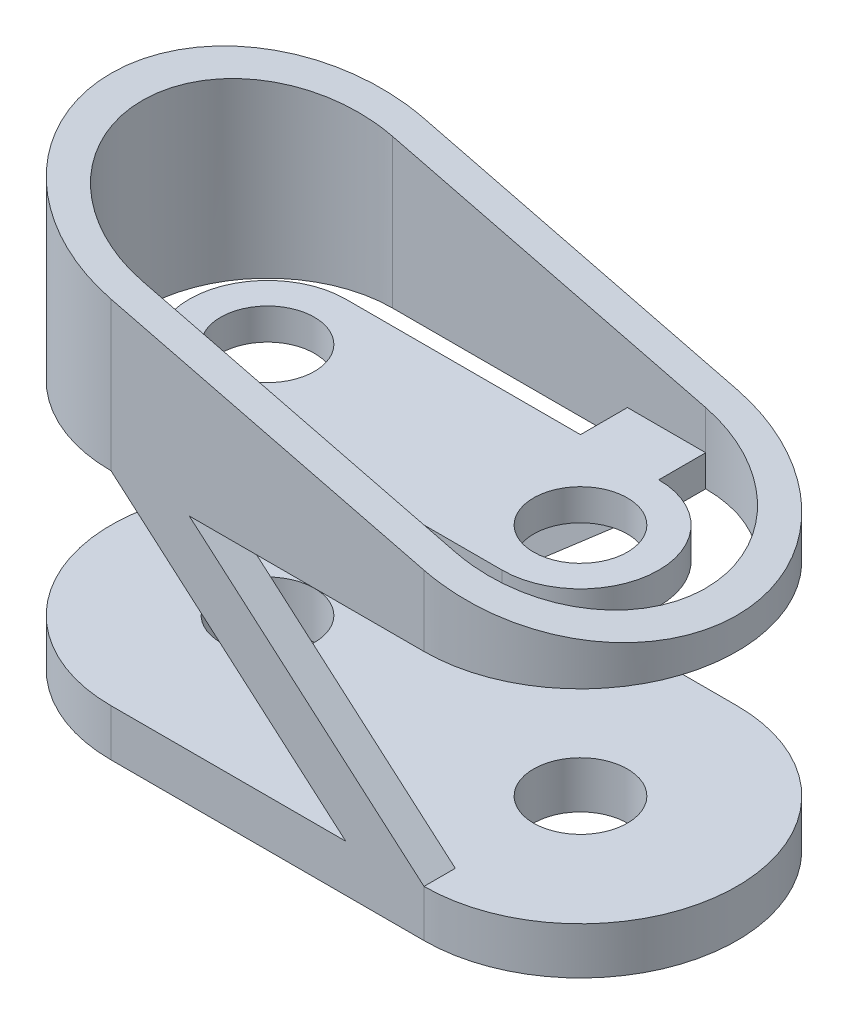
ISO-10303-21;
HEADER;
FILE_DESCRIPTION(('STEP AP214'),'2;1');
FILE_NAME('part.step','',(''),(''),'','','');
FILE_SCHEMA(('AUTOMOTIVE_DESIGN { 1 0 10303 214 1 1 1 1 }'));
ENDSEC;
DATA;
#1=APPLICATION_CONTEXT('core data for automotive mechanical design processes');
#2=APPLICATION_PROTOCOL_DEFINITION('international standard','automotive_design',2000,#1);
#3=PRODUCT_CONTEXT('',#1,'mechanical');
#4=PRODUCT('Part','Part','',(#3));
#5=PRODUCT_RELATED_PRODUCT_CATEGORY('part','',(#4));
#6=PRODUCT_DEFINITION_FORMATION('','',#4);
#7=PRODUCT_DEFINITION_CONTEXT('part definition',#1,'design');
#8=PRODUCT_DEFINITION('design','',#6,#7);
#9=PRODUCT_DEFINITION_SHAPE('','',#8);
#10=(LENGTH_UNIT() NAMED_UNIT(*) SI_UNIT(.MILLI.,.METRE.));
#11=(NAMED_UNIT(*) PLANE_ANGLE_UNIT() SI_UNIT($,.RADIAN.));
#12=(NAMED_UNIT(*) SI_UNIT($,.STERADIAN.) SOLID_ANGLE_UNIT());
#13=UNCERTAINTY_MEASURE_WITH_UNIT(LENGTH_MEASURE(1.E-05),#10,'distance_accuracy_value','');
#14=(GEOMETRIC_REPRESENTATION_CONTEXT(3) GLOBAL_UNCERTAINTY_ASSIGNED_CONTEXT((#13)) GLOBAL_UNIT_ASSIGNED_CONTEXT((#10,
#11,#12)) REPRESENTATION_CONTEXT('',''));
#15=CARTESIAN_POINT('',(0.,0.,0.));
#16=DIRECTION('',(0.,0.,1.));
#17=DIRECTION('',(1.,0.,0.));
#18=AXIS2_PLACEMENT_3D('',#15,#16,#17);
#19=CARTESIAN_POINT('',(100.,105.,-40.));
#20=DIRECTION('',(0.,0.,1.));
#21=DIRECTION('',(1.,0.,0.));
#22=AXIS2_PLACEMENT_3D('',#19,#20,#21);
#23=PLANE('',#22);
#24=DIRECTION('',(0.970142500145332,-0.242535625036333,0.));
#25=VECTOR('',#24,1.);
#26=CARTESIAN_POINT('',(99.4117647058824,102.647058823529,-40.));
#27=LINE('',#26,#25);
#28=CARTESIAN_POINT('',(0.,127.5,-40.));
#29=VERTEX_POINT('',#28);
#30=CARTESIAN_POINT('',(100.,102.5,-40.));
#31=VERTEX_POINT('',#30);
#32=EDGE_CURVE('E559',#29,#31,#27,.T.);
#33=ORIENTED_EDGE('',*,*,#32,.F.);
#34=DIRECTION('',(0.,-1.,0.));
#35=VECTOR('',#34,1.);
#36=CARTESIAN_POINT('',(0.,105.,-40.));
#37=LINE('',#36,#35);
#38=CARTESIAN_POINT('',(0.,80.,-40.));
#39=VERTEX_POINT('',#38);
#40=EDGE_CURVE('E501',#29,#39,#37,.T.);
#41=ORIENTED_EDGE('',*,*,#40,.T.);
#42=DIRECTION('',(1.,0.,0.));
#43=VECTOR('',#42,1.);
#44=CARTESIAN_POINT('',(100.,80.,-40.));
#45=LINE('',#44,#43);
#46=CARTESIAN_POINT('',(75.,80.,-40.));
#47=VERTEX_POINT('',#46);
#48=EDGE_CURVE('E494',#39,#47,#45,.T.);
#49=ORIENTED_EDGE('',*,*,#48,.T.);
#50=DIRECTION('',(0.,-1.,0.));
#51=VECTOR('',#50,1.);
#52=CARTESIAN_POINT('',(75.,105.,-40.));
#53=LINE('',#52,#51);
#54=CARTESIAN_POINT('',(75.,90.,-40.));
#55=VERTEX_POINT('',#54);
#56=EDGE_CURVE('E530',#55,#47,#53,.T.);
#57=ORIENTED_EDGE('',*,*,#56,.F.);
#58=DIRECTION('',(-1.,0.,0.));
#59=VECTOR('',#58,1.);
#60=CARTESIAN_POINT('',(0.,90.,-40.));
#61=LINE('',#60,#59);
#62=CARTESIAN_POINT('',(100.,90.,-40.));
#63=VERTEX_POINT('',#62);
#64=EDGE_CURVE('E553',#63,#55,#61,.T.);
#65=ORIENTED_EDGE('',*,*,#64,.F.);
#66=DIRECTION('',(0.,-1.,0.));
#67=VECTOR('',#66,1.);
#68=CARTESIAN_POINT('',(100.,140.,-40.));
#69=LINE('',#68,#67);
#70=EDGE_CURVE('E541',#31,#63,#69,.T.);
#71=ORIENTED_EDGE('',*,*,#70,.F.);
#72=EDGE_LOOP('',(#33,#41,#49,#57,#65,#71));
#73=FACE_BOUND('',#72,.T.);
#74=ADVANCED_FACE('F126',(#73),#23,.T.);
#75=CARTESIAN_POINT('',(100.,80.,0.));
#76=DIRECTION('',(0.,1.,0.));
#77=DIRECTION('',(0.,0.,1.));
#78=AXIS2_PLACEMENT_3D('',#75,#76,#77);
#79=PLANE('',#78);
#80=CARTESIAN_POINT('',(100.,80.,0.));
#81=DIRECTION('',(0.,1.,0.));
#82=DIRECTION('',(0.,0.,1.));
#83=AXIS2_PLACEMENT_3D('',#80,#81,#82);
#84=CIRCLE('',#83,40.);
#85=CARTESIAN_POINT('',(100.,80.,-40.));
#86=VERTEX_POINT('',#85);
#87=CARTESIAN_POINT('',(100.,80.,40.));
#88=VERTEX_POINT('',#87);
#89=EDGE_CURVE('E493',#86,#88,#84,.F.);
#90=ORIENTED_EDGE('',*,*,#89,.F.);
#91=DIRECTION('',(0.,0.,-1.));
#92=VECTOR('',#91,1.);
#93=CARTESIAN_POINT('',(100.,80.,-40.));
#94=LINE('',#93,#92);
#95=CARTESIAN_POINT('',(100.,80.,-50.));
#96=VERTEX_POINT('',#95);
#97=EDGE_CURVE('E517',#86,#96,#94,.T.);
#98=ORIENTED_EDGE('',*,*,#97,.T.);
#99=CARTESIAN_POINT('',(100.,80.,0.));
#100=DIRECTION('',(0.,1.,0.));
#101=DIRECTION('',(0.,0.,1.));
#102=AXIS2_PLACEMENT_3D('',#99,#100,#101);
#103=CIRCLE('',#102,50.);
#104=CARTESIAN_POINT('',(100.,80.,50.));
#105=VERTEX_POINT('',#104);
#106=EDGE_CURVE('E482',#105,#96,#103,.T.);
#107=ORIENTED_EDGE('',*,*,#106,.F.);
#108=DIRECTION('',(1.,0.,0.));
#109=VECTOR('',#108,1.);
#110=CARTESIAN_POINT('',(0.,80.,50.));
#111=LINE('',#110,#109);
#112=CARTESIAN_POINT('',(25.0000000000005,80.,50.));
#113=VERTEX_POINT('',#112);
#114=EDGE_CURVE('E485',#113,#105,#111,.T.);
#115=ORIENTED_EDGE('',*,*,#114,.F.);
#116=DIRECTION('',(0.,0.,1.));
#117=VECTOR('',#116,1.);
#118=CARTESIAN_POINT('',(25.,80.,40.));
#119=LINE('',#118,#117);
#120=CARTESIAN_POINT('',(25.0000000000005,80.,40.));
#121=VERTEX_POINT('',#120);
#122=EDGE_CURVE('E454',#121,#113,#119,.T.);
#123=ORIENTED_EDGE('',*,*,#122,.F.);
#124=DIRECTION('',(1.,0.,0.));
#125=VECTOR('',#124,1.);
#126=CARTESIAN_POINT('',(100.,80.,40.));
#127=LINE('',#126,#125);
#128=EDGE_CURVE('E486',#121,#88,#127,.T.);
#129=ORIENTED_EDGE('',*,*,#128,.T.);
#130=EDGE_LOOP('',(#90,#98,#107,#115,#123,#129));
#131=FACE_BOUND('',#130,.T.);
#132=ADVANCED_FACE('F594',(#131),#79,.F.);
#133=CARTESIAN_POINT('',(0.,80.,0.));
#134=DIRECTION('',(0.,1.,0.));
#135=DIRECTION('',(0.,0.,1.));
#136=AXIS2_PLACEMENT_3D('',#133,#134,#135);
#137=PLANE('',#136);
#138=CARTESIAN_POINT('',(0.,80.,0.));
#139=DIRECTION('',(0.,1.,0.));
#140=DIRECTION('',(0.,0.,1.));
#141=AXIS2_PLACEMENT_3D('',#138,#139,#140);
#142=CIRCLE('',#141,15.);
#143=CARTESIAN_POINT('',(0.,80.,15.));
#144=VERTEX_POINT('',#143);
#145=EDGE_CURVE('E333',#144,#144,#142,.T.);
#146=ORIENTED_EDGE('',*,*,#145,.T.);
#147=EDGE_LOOP('',(#146));
#148=FACE_BOUND('',#147,.T.);
#149=CARTESIAN_POINT('',(100.,80.,0.));
#150=DIRECTION('',(0.,1.,0.));
#151=DIRECTION('',(0.,0.,1.));
#152=AXIS2_PLACEMENT_3D('',#149,#150,#151);
#153=CIRCLE('',#152,15.);
#154=CARTESIAN_POINT('',(100.,80.,15.));
#155=VERTEX_POINT('',#154);
#156=EDGE_CURVE('E325',#155,#155,#153,.T.);
#157=ORIENTED_EDGE('',*,*,#156,.T.);
#158=EDGE_LOOP('',(#157));
#159=FACE_BOUND('',#158,.T.);
#160=DIRECTION('',(0.,0.,-1.));
#161=VECTOR('',#160,1.);
#162=CARTESIAN_POINT('',(25.0000000000005,80.,50.));
#163=LINE('',#162,#161);
#164=CARTESIAN_POINT('',(25.0000000000005,80.,25.));
#165=VERTEX_POINT('',#164);
#166=EDGE_CURVE('E316',#121,#165,#163,.T.);
#167=ORIENTED_EDGE('',*,*,#166,.F.);
#168=DIRECTION('',(-1.,0.,0.));
#169=VECTOR('',#168,1.);
#170=CARTESIAN_POINT('',(0.,80.,40.));
#171=LINE('',#170,#169);
#172=CARTESIAN_POINT('',(5.2372220082647E-13,80.,40.));
#173=VERTEX_POINT('',#172);
#174=EDGE_CURVE('E383',#121,#173,#171,.T.);
#175=ORIENTED_EDGE('',*,*,#174,.T.);
#176=DIRECTION('',(0.,0.,1.));
#177=VECTOR('',#176,1.);
#178=CARTESIAN_POINT('',(5.2372220082647E-13,80.,50.));
#179=LINE('',#178,#177);
#180=CARTESIAN_POINT('',(5.2372220082647E-13,80.,25.));
#181=VERTEX_POINT('',#180);
#182=EDGE_CURVE('E321',#181,#173,#179,.T.);
#183=ORIENTED_EDGE('',*,*,#182,.F.);
#184=CARTESIAN_POINT('',(0.,80.,0.));
#185=DIRECTION('',(0.,1.,0.));
#186=DIRECTION('',(0.,0.,1.));
#187=AXIS2_PLACEMENT_3D('',#184,#185,#186);
#188=CIRCLE('',#187,25.);
#189=CARTESIAN_POINT('',(0.,80.,-25.));
#190=VERTEX_POINT('',#189);
#191=EDGE_CURVE('E352',#190,#181,#188,.T.);
#192=ORIENTED_EDGE('',*,*,#191,.F.);
#193=DIRECTION('',(-1.,0.,0.));
#194=VECTOR('',#193,1.);
#195=CARTESIAN_POINT('',(100.,80.,-25.));
#196=LINE('',#195,#194);
#197=CARTESIAN_POINT('',(75.,80.,-25.));
#198=VERTEX_POINT('',#197);
#199=EDGE_CURVE('E358',#198,#190,#196,.T.);
#200=ORIENTED_EDGE('',*,*,#199,.F.);
#201=DIRECTION('',(0.,0.,1.));
#202=VECTOR('',#201,1.);
#203=CARTESIAN_POINT('',(75.,80.,-50.));
#204=LINE('',#203,#202);
#205=EDGE_CURVE('E540',#47,#198,#204,.T.);
#206=ORIENTED_EDGE('',*,*,#205,.F.);
#207=DIRECTION('',(1.,0.,0.));
#208=VECTOR('',#207,1.);
#209=CARTESIAN_POINT('',(100.,80.,-40.));
#210=LINE('',#209,#208);
#211=EDGE_CURVE('E531',#47,#86,#210,.T.);
#212=ORIENTED_EDGE('',*,*,#211,.T.);
#213=DIRECTION('',(0.,0.,-1.));
#214=VECTOR('',#213,1.);
#215=CARTESIAN_POINT('',(100.,80.,-50.));
#216=LINE('',#215,#214);
#217=CARTESIAN_POINT('',(100.,80.,-25.));
#218=VERTEX_POINT('',#217);
#219=EDGE_CURVE('E542',#218,#86,#216,.T.);
#220=ORIENTED_EDGE('',*,*,#219,.F.);
#221=CARTESIAN_POINT('',(100.,80.,0.));
#222=DIRECTION('',(0.,1.,0.));
#223=DIRECTION('',(0.,0.,1.));
#224=AXIS2_PLACEMENT_3D('',#221,#222,#223);
#225=CIRCLE('',#224,25.);
#226=CARTESIAN_POINT('',(100.,80.,25.));
#227=VERTEX_POINT('',#226);
#228=EDGE_CURVE('E341',#227,#218,#225,.T.);
#229=ORIENTED_EDGE('',*,*,#228,.F.);
#230=DIRECTION('',(-1.,0.,0.));
#231=VECTOR('',#230,1.);
#232=CARTESIAN_POINT('',(100.,80.,25.));
#233=LINE('',#232,#231);
#234=EDGE_CURVE('E340',#227,#165,#233,.T.);
#235=ORIENTED_EDGE('',*,*,#234,.T.);
#236=EDGE_LOOP('',(#167,#175,#183,#192,#200,#206,#212,#220,#229,#235));
#237=FACE_BOUND('',#236,.T.);
#238=ADVANCED_FACE('F385',(#148,#159,#237),#137,.F.);
#239=CARTESIAN_POINT('',(0.,90.,0.));
#240=DIRECTION('',(0.,1.,0.));
#241=DIRECTION('',(0.,0.,1.));
#242=AXIS2_PLACEMENT_3D('',#239,#240,#241);
#243=PLANE('',#242);
#244=DIRECTION('',(-1.,0.,0.));
#245=VECTOR('',#244,1.);
#246=CARTESIAN_POINT('',(0.,90.,40.));
#247=LINE('',#246,#245);
#248=CARTESIAN_POINT('',(25.0000000000005,90.,40.));
#249=VERTEX_POINT('',#248);
#250=CARTESIAN_POINT('',(5.2372220082647E-13,90.,40.));
#251=VERTEX_POINT('',#250);
#252=EDGE_CURVE('E12',#249,#251,#247,.T.);
#253=ORIENTED_EDGE('',*,*,#252,.F.);
#254=DIRECTION('',(0.,0.,-1.));
#255=VECTOR('',#254,1.);
#256=CARTESIAN_POINT('',(25.0000000000005,90.,50.));
#257=LINE('',#256,#255);
#258=CARTESIAN_POINT('',(25.0000000000005,90.,25.));
#259=VERTEX_POINT('',#258);
#260=EDGE_CURVE('E387',#249,#259,#257,.T.);
#261=ORIENTED_EDGE('',*,*,#260,.T.);
#262=DIRECTION('',(-1.,0.,0.));
#263=VECTOR('',#262,1.);
#264=CARTESIAN_POINT('',(100.,90.,25.));
#265=LINE('',#264,#263);
#266=CARTESIAN_POINT('',(100.,90.,25.));
#267=VERTEX_POINT('',#266);
#268=EDGE_CURVE('E338',#267,#259,#265,.T.);
#269=ORIENTED_EDGE('',*,*,#268,.F.);
#270=CARTESIAN_POINT('',(100.,90.,0.));
#271=DIRECTION('',(0.,1.,0.));
#272=DIRECTION('',(0.,0.,1.));
#273=AXIS2_PLACEMENT_3D('',#270,#271,#272);
#274=CIRCLE('',#273,25.);
#275=CARTESIAN_POINT('',(100.,90.,-25.));
#276=VERTEX_POINT('',#275);
#277=EDGE_CURVE('E348',#267,#276,#274,.T.);
#278=ORIENTED_EDGE('',*,*,#277,.T.);
#279=DIRECTION('',(0.,0.,-1.));
#280=VECTOR('',#279,1.);
#281=CARTESIAN_POINT('',(100.,90.,-50.));
#282=LINE('',#281,#280);
#283=EDGE_CURVE('E545',#276,#63,#282,.T.);
#284=ORIENTED_EDGE('',*,*,#283,.T.);
#285=ORIENTED_EDGE('',*,*,#64,.T.);
#286=DIRECTION('',(0.,0.,1.));
#287=VECTOR('',#286,1.);
#288=CARTESIAN_POINT('',(75.,90.,-50.));
#289=LINE('',#288,#287);
#290=CARTESIAN_POINT('',(75.,90.,-25.));
#291=VERTEX_POINT('',#290);
#292=EDGE_CURVE('E539',#55,#291,#289,.T.);
#293=ORIENTED_EDGE('',*,*,#292,.T.);
#294=DIRECTION('',(-1.,0.,0.));
#295=VECTOR('',#294,1.);
#296=CARTESIAN_POINT('',(100.,90.,-25.));
#297=LINE('',#296,#295);
#298=CARTESIAN_POINT('',(0.,90.,-25.));
#299=VERTEX_POINT('',#298);
#300=EDGE_CURVE('E347',#291,#299,#297,.T.);
#301=ORIENTED_EDGE('',*,*,#300,.T.);
#302=CARTESIAN_POINT('',(0.,90.,0.));
#303=DIRECTION('',(0.,1.,0.));
#304=DIRECTION('',(0.,0.,1.));
#305=AXIS2_PLACEMENT_3D('',#302,#303,#304);
#306=CIRCLE('',#305,25.);
#307=CARTESIAN_POINT('',(0.,90.,25.));
#308=VERTEX_POINT('',#307);
#309=EDGE_CURVE('E344',#299,#308,#306,.T.);
#310=ORIENTED_EDGE('',*,*,#309,.T.);
#311=DIRECTION('',(0.,0.,1.));
#312=VECTOR('',#311,1.);
#313=CARTESIAN_POINT('',(5.2372220082647E-13,90.,50.));
#314=LINE('',#313,#312);
#315=EDGE_CURVE('E376',#308,#251,#314,.T.);
#316=ORIENTED_EDGE('',*,*,#315,.T.);
#317=EDGE_LOOP('',(#253,#261,#269,#278,#284,#285,#293,#301,#310,#316));
#318=FACE_BOUND('',#317,.T.);
#319=CARTESIAN_POINT('',(100.,90.,0.));
#320=DIRECTION('',(0.,1.,0.));
#321=DIRECTION('',(0.,0.,1.));
#322=AXIS2_PLACEMENT_3D('',#319,#320,#321);
#323=CIRCLE('',#322,15.);
#324=CARTESIAN_POINT('',(100.,90.,15.));
#325=VERTEX_POINT('',#324);
#326=EDGE_CURVE('E328',#325,#325,#323,.T.);
#327=ORIENTED_EDGE('',*,*,#326,.F.);
#328=EDGE_LOOP('',(#327));
#329=FACE_BOUND('',#328,.T.);
#330=CARTESIAN_POINT('',(0.,90.,0.));
#331=DIRECTION('',(0.,1.,0.));
#332=DIRECTION('',(0.,0.,1.));
#333=AXIS2_PLACEMENT_3D('',#330,#331,#332);
#334=CIRCLE('',#333,15.);
#335=CARTESIAN_POINT('',(0.,90.,15.));
#336=VERTEX_POINT('',#335);
#337=EDGE_CURVE('E332',#336,#336,#334,.T.);
#338=ORIENTED_EDGE('',*,*,#337,.F.);
#339=EDGE_LOOP('',(#338));
#340=FACE_BOUND('',#339,.T.);
#341=ADVANCED_FACE('F603',(#318,#329,#340),#243,.T.);
#342=CARTESIAN_POINT('',(100.,90.,25.));
#343=DIRECTION('',(0.,0.,1.));
#344=DIRECTION('',(1.,0.,0.));
#345=AXIS2_PLACEMENT_3D('',#342,#343,#344);
#346=PLANE('',#345);
#347=DIRECTION('',(0.,1.,0.));
#348=VECTOR('',#347,1.);
#349=CARTESIAN_POINT('',(25.0000000000005,80.,25.));
#350=LINE('',#349,#348);
#351=EDGE_CURVE('E319',#165,#259,#350,.T.);
#352=ORIENTED_EDGE('',*,*,#351,.F.);
#353=ORIENTED_EDGE('',*,*,#234,.F.);
#354=DIRECTION('',(0.,-1.,0.));
#355=VECTOR('',#354,1.);
#356=CARTESIAN_POINT('',(100.,90.,25.));
#357=LINE('',#356,#355);
#358=EDGE_CURVE('E359',#267,#227,#357,.T.);
#359=ORIENTED_EDGE('',*,*,#358,.F.);
#360=ORIENTED_EDGE('',*,*,#268,.T.);
#361=EDGE_LOOP('',(#352,#353,#359,#360));
#362=FACE_BOUND('',#361,.T.);
#363=ADVANCED_FACE('F132',(#362),#346,.T.);
#364=CARTESIAN_POINT('',(100.,90.,0.));
#365=DIRECTION('',(0.,-1.,0.));
#366=DIRECTION('',(0.,0.,-1.));
#367=AXIS2_PLACEMENT_3D('',#364,#365,#366);
#368=CYLINDRICAL_SURFACE('',#367,25.);
#369=ORIENTED_EDGE('',*,*,#228,.T.);
#370=DIRECTION('',(0.,-1.,0.));
#371=VECTOR('',#370,1.);
#372=CARTESIAN_POINT('',(100.,90.,-25.));
#373=LINE('',#372,#371);
#374=EDGE_CURVE('E365',#276,#218,#373,.T.);
#375=ORIENTED_EDGE('',*,*,#374,.F.);
#376=ORIENTED_EDGE('',*,*,#277,.F.);
#377=ORIENTED_EDGE('',*,*,#358,.T.);
#378=EDGE_LOOP('',(#369,#375,#376,#377));
#379=FACE_BOUND('',#378,.T.);
#380=ADVANCED_FACE('F615',(#379),#368,.T.);
#381=CARTESIAN_POINT('',(100.,90.,-25.));
#382=DIRECTION('',(0.,0.,1.));
#383=DIRECTION('',(1.,0.,0.));
#384=AXIS2_PLACEMENT_3D('',#381,#382,#383);
#385=PLANE('',#384);
#386=ORIENTED_EDGE('',*,*,#300,.F.);
#387=DIRECTION('',(0.,1.,0.));
#388=VECTOR('',#387,1.);
#389=CARTESIAN_POINT('',(75.,80.,-25.));
#390=LINE('',#389,#388);
#391=EDGE_CURVE('E533',#198,#291,#390,.T.);
#392=ORIENTED_EDGE('',*,*,#391,.F.);
#393=ORIENTED_EDGE('',*,*,#199,.T.);
#394=DIRECTION('',(0.,-1.,0.));
#395=VECTOR('',#394,1.);
#396=CARTESIAN_POINT('',(0.,90.,-25.));
#397=LINE('',#396,#395);
#398=EDGE_CURVE('E364',#299,#190,#397,.T.);
#399=ORIENTED_EDGE('',*,*,#398,.F.);
#400=EDGE_LOOP('',(#386,#392,#393,#399));
#401=FACE_BOUND('',#400,.T.);
#402=ADVANCED_FACE('F619',(#401),#385,.F.);
#403=CARTESIAN_POINT('',(0.,90.,0.));
#404=DIRECTION('',(0.,-1.,0.));
#405=DIRECTION('',(0.,0.,-1.));
#406=AXIS2_PLACEMENT_3D('',#403,#404,#405);
#407=CYLINDRICAL_SURFACE('',#406,25.);
#408=ORIENTED_EDGE('',*,*,#191,.T.);
#409=DIRECTION('',(0.,-1.,0.));
#410=VECTOR('',#409,1.);
#411=CARTESIAN_POINT('',(0.,90.,25.));
#412=LINE('',#411,#410);
#413=EDGE_CURVE('E353',#308,#181,#412,.T.);
#414=ORIENTED_EDGE('',*,*,#413,.F.);
#415=ORIENTED_EDGE('',*,*,#309,.F.);
#416=ORIENTED_EDGE('',*,*,#398,.T.);
#417=EDGE_LOOP('',(#408,#414,#415,#416));
#418=FACE_BOUND('',#417,.T.);
#419=ADVANCED_FACE('F625',(#418),#407,.T.);
#420=CARTESIAN_POINT('',(0.,90.,0.));
#421=DIRECTION('',(0.,-1.,0.));
#422=DIRECTION('',(0.,0.,-1.));
#423=AXIS2_PLACEMENT_3D('',#420,#421,#422);
#424=CYLINDRICAL_SURFACE('',#423,15.);
#425=ORIENTED_EDGE('',*,*,#337,.T.);
#426=EDGE_LOOP('',(#425));
#427=FACE_BOUND('',#426,.T.);
#428=ORIENTED_EDGE('',*,*,#145,.F.);
#429=EDGE_LOOP('',(#428));
#430=FACE_BOUND('',#429,.T.);
#431=ADVANCED_FACE('F624',(#427,#430),#424,.F.);
#432=CARTESIAN_POINT('',(100.,90.,0.));
#433=DIRECTION('',(0.,-1.,0.));
#434=DIRECTION('',(0.,0.,-1.));
#435=AXIS2_PLACEMENT_3D('',#432,#433,#434);
#436=CYLINDRICAL_SURFACE('',#435,15.);
#437=ORIENTED_EDGE('',*,*,#326,.T.);
#438=EDGE_LOOP('',(#437));
#439=FACE_BOUND('',#438,.T.);
#440=ORIENTED_EDGE('',*,*,#156,.F.);
#441=EDGE_LOOP('',(#440));
#442=FACE_BOUND('',#441,.T.);
#443=ADVANCED_FACE('F629',(#439,#442),#436,.F.);
#444=CARTESIAN_POINT('',(5.2372220082647E-13,80.,50.));
#445=DIRECTION('',(-1.,0.,0.));
#446=DIRECTION('',(0.,0.,1.));
#447=AXIS2_PLACEMENT_3D('',#444,#445,#446);
#448=PLANE('',#447);
#449=DIRECTION('',(0.,-1.,0.));
#450=VECTOR('',#449,1.);
#451=CARTESIAN_POINT('',(0.,90.,40.));
#452=LINE('',#451,#450);
#453=EDGE_CURVE('E472',#251,#173,#452,.T.);
#454=ORIENTED_EDGE('',*,*,#453,.F.);
#455=ORIENTED_EDGE('',*,*,#315,.F.);
#456=ORIENTED_EDGE('',*,*,#413,.T.);
#457=ORIENTED_EDGE('',*,*,#182,.T.);
#458=EDGE_LOOP('',(#454,#455,#456,#457));
#459=FACE_BOUND('',#458,.T.);
#460=ADVANCED_FACE('F373',(#459),#448,.T.);
#461=CARTESIAN_POINT('',(25.0000000000005,80.,50.));
#462=DIRECTION('',(1.,0.,0.));
#463=DIRECTION('',(0.,0.,-1.));
#464=AXIS2_PLACEMENT_3D('',#461,#462,#463);
#465=PLANE('',#464);
#466=DIRECTION('',(0.,1.,0.));
#467=VECTOR('',#466,1.);
#468=CARTESIAN_POINT('',(25.0000000000005,80.,40.));
#469=LINE('',#468,#467);
#470=EDGE_CURVE('E133',#121,#249,#469,.T.);
#471=ORIENTED_EDGE('',*,*,#470,.F.);
#472=ORIENTED_EDGE('',*,*,#166,.T.);
#473=ORIENTED_EDGE('',*,*,#351,.T.);
#474=ORIENTED_EDGE('',*,*,#260,.F.);
#475=EDGE_LOOP('',(#471,#472,#473,#474));
#476=FACE_BOUND('',#475,.T.);
#477=ADVANCED_FACE('F738',(#476),#465,.T.);
#478=CARTESIAN_POINT('',(5.2372220082647E-13,80.,50.));
#479=DIRECTION('',(0.,0.,1.));
#480=DIRECTION('',(1.,0.,0.));
#481=AXIS2_PLACEMENT_3D('',#478,#479,#480);
#482=PLANE('',#481);
#483=DIRECTION('',(0.970142500145332,-0.242535625036333,0.));
#484=VECTOR('',#483,1.);
#485=CARTESIAN_POINT('',(150.,90.,50.));
#486=LINE('',#485,#484);
#487=CARTESIAN_POINT('',(0.,127.5,50.));
#488=VERTEX_POINT('',#487);
#489=CARTESIAN_POINT('',(100.,102.5,50.));
#490=VERTEX_POINT('',#489);
#491=EDGE_CURVE('E300',#488,#490,#486,.T.);
#492=ORIENTED_EDGE('',*,*,#491,.F.);
#493=DIRECTION('',(0.,1.,0.));
#494=VECTOR('',#493,1.);
#495=CARTESIAN_POINT('',(5.2372220082647E-13,80.,50.));
#496=LINE('',#495,#494);
#497=CARTESIAN_POINT('',(5.2372220082647E-13,80.,50.));
#498=VERTEX_POINT('',#497);
#499=EDGE_CURVE('E308',#498,#488,#496,.T.);
#500=ORIENTED_EDGE('',*,*,#499,.F.);
#501=DIRECTION('',(0.755689082789818,-0.654930538417842,0.));
#502=VECTOR('',#501,1.);
#503=CARTESIAN_POINT('',(0.,80.,50.));
#504=LINE('',#503,#502);
#505=CARTESIAN_POINT('',(75.,15.,50.));
#506=VERTEX_POINT('',#505);
#507=EDGE_CURVE('E465',#498,#506,#504,.T.);
#508=ORIENTED_EDGE('',*,*,#507,.T.);
#509=DIRECTION('',(1.,0.,0.));
#510=VECTOR('',#509,1.);
#511=CARTESIAN_POINT('',(0.,15.,50.));
#512=LINE('',#511,#510);
#513=CARTESIAN_POINT('',(0.,15.,50.));
#514=VERTEX_POINT('',#513);
#515=EDGE_CURVE('E414',#514,#506,#512,.T.);
#516=ORIENTED_EDGE('',*,*,#515,.F.);
#517=DIRECTION('',(0.,-1.,0.));
#518=VECTOR('',#517,1.);
#519=CARTESIAN_POINT('',(0.,15.,50.));
#520=LINE('',#519,#518);
#521=CARTESIAN_POINT('',(0.,0.,50.));
#522=VERTEX_POINT('',#521);
#523=EDGE_CURVE('E393',#514,#522,#520,.T.);
#524=ORIENTED_EDGE('',*,*,#523,.T.);
#525=DIRECTION('',(1.,0.,0.));
#526=VECTOR('',#525,1.);
#527=CARTESIAN_POINT('',(0.,0.,50.));
#528=LINE('',#527,#526);
#529=CARTESIAN_POINT('',(100.,0.,50.));
#530=VERTEX_POINT('',#529);
#531=EDGE_CURVE('E430',#522,#530,#528,.T.);
#532=ORIENTED_EDGE('',*,*,#531,.T.);
#533=DIRECTION('',(0.,-1.,0.));
#534=VECTOR('',#533,1.);
#535=CARTESIAN_POINT('',(100.,15.,50.));
#536=LINE('',#535,#534);
#537=CARTESIAN_POINT('',(100.,15.,50.));
#538=VERTEX_POINT('',#537);
#539=EDGE_CURVE('E399',#538,#530,#536,.T.);
#540=ORIENTED_EDGE('',*,*,#539,.F.);
#541=DIRECTION('',(-0.755689082789818,0.654930538417842,0.));
#542=VECTOR('',#541,1.);
#543=CARTESIAN_POINT('',(25.,80.,50.));
#544=LINE('',#543,#542);
#545=EDGE_CURVE('E464',#538,#113,#544,.T.);
#546=ORIENTED_EDGE('',*,*,#545,.T.);
#547=ORIENTED_EDGE('',*,*,#114,.T.);
#548=DIRECTION('',(0.,1.,0.));
#549=VECTOR('',#548,1.);
#550=CARTESIAN_POINT('',(100.,80.,50.));
#551=LINE('',#550,#549);
#552=EDGE_CURVE('E311',#105,#490,#551,.T.);
#553=ORIENTED_EDGE('',*,*,#552,.T.);
#554=EDGE_LOOP('',(#492,#500,#508,#516,#524,#532,#540,#546,#547,#553));
#555=FACE_BOUND('',#554,.T.);
#556=ADVANCED_FACE('F306',(#555),#482,.T.);
#557=CARTESIAN_POINT('',(0.,0.,40.));
#558=DIRECTION('',(0.,0.,-1.));
#559=DIRECTION('',(-1.,0.,0.));
#560=AXIS2_PLACEMENT_3D('',#557,#558,#559);
#561=PLANE('',#560);
#562=ORIENTED_EDGE('',*,*,#174,.F.);
#563=DIRECTION('',(-0.755689082789818,0.654930538417842,0.));
#564=VECTOR('',#563,1.);
#565=CARTESIAN_POINT('',(25.,80.,40.));
#566=LINE('',#565,#564);
#567=CARTESIAN_POINT('',(100.,15.,40.));
#568=VERTEX_POINT('',#567);
#569=EDGE_CURVE('E462',#568,#121,#566,.T.);
#570=ORIENTED_EDGE('',*,*,#569,.F.);
#571=DIRECTION('',(-1.,0.,0.));
#572=VECTOR('',#571,1.);
#573=CARTESIAN_POINT('',(100.,15.,40.));
#574=LINE('',#573,#572);
#575=CARTESIAN_POINT('',(75.,15.,40.));
#576=VERTEX_POINT('',#575);
#577=EDGE_CURVE('E443',#568,#576,#574,.T.);
#578=ORIENTED_EDGE('',*,*,#577,.T.);
#579=DIRECTION('',(0.755689082789818,-0.654930538417842,0.));
#580=VECTOR('',#579,1.);
#581=CARTESIAN_POINT('',(0.,80.,40.));
#582=LINE('',#581,#580);
#583=EDGE_CURVE('E451',#173,#576,#582,.T.);
#584=ORIENTED_EDGE('',*,*,#583,.F.);
#585=EDGE_LOOP('',(#562,#570,#578,#584));
#586=FACE_BOUND('',#585,.T.);
#587=ADVANCED_FACE('F717',(#586),#561,.T.);
#588=CARTESIAN_POINT('',(100.,15.,0.));
#589=DIRECTION('',(0.,1.,0.));
#590=DIRECTION('',(0.,0.,1.));
#591=AXIS2_PLACEMENT_3D('',#588,#589,#590);
#592=PLANE('',#591);
#593=DIRECTION('',(0.,0.,-1.));
#594=VECTOR('',#593,1.);
#595=CARTESIAN_POINT('',(25.,15.,-40.));
#596=LINE('',#595,#594);
#597=CARTESIAN_POINT('',(25.,15.,-40.));
#598=VERTEX_POINT('',#597);
#599=CARTESIAN_POINT('',(25.,15.,-50.));
#600=VERTEX_POINT('',#599);
#601=EDGE_CURVE('E508',#598,#600,#596,.T.);
#602=ORIENTED_EDGE('',*,*,#601,.F.);
#603=DIRECTION('',(1.,0.,0.));
#604=VECTOR('',#603,1.);
#605=CARTESIAN_POINT('',(100.,15.,-40.));
#606=LINE('',#605,#604);
#607=CARTESIAN_POINT('',(0.,15.,-40.));
#608=VERTEX_POINT('',#607);
#609=EDGE_CURVE('E502',#608,#598,#606,.T.);
#610=ORIENTED_EDGE('',*,*,#609,.F.);
#611=DIRECTION('',(0.,0.,-1.));
#612=VECTOR('',#611,1.);
#613=CARTESIAN_POINT('',(0.,15.,-40.));
#614=LINE('',#613,#612);
#615=CARTESIAN_POINT('',(0.,15.,-50.));
#616=VERTEX_POINT('',#615);
#617=EDGE_CURVE('E509',#608,#616,#614,.T.);
#618=ORIENTED_EDGE('',*,*,#617,.T.);
#619=CARTESIAN_POINT('',(0.,15.,0.));
#620=DIRECTION('',(0.,1.,0.));
#621=DIRECTION('',(0.,0.,1.));
#622=AXIS2_PLACEMENT_3D('',#619,#620,#621);
#623=CIRCLE('',#622,50.);
#624=EDGE_CURVE('E406',#616,#514,#623,.T.);
#625=ORIENTED_EDGE('',*,*,#624,.T.);
#626=ORIENTED_EDGE('',*,*,#515,.T.);
#627=DIRECTION('',(0.,0.,1.));
#628=VECTOR('',#627,1.);
#629=CARTESIAN_POINT('',(75.,15.,40.));
#630=LINE('',#629,#628);
#631=EDGE_CURVE('E446',#576,#506,#630,.T.);
#632=ORIENTED_EDGE('',*,*,#631,.F.);
#633=ORIENTED_EDGE('',*,*,#577,.F.);
#634=DIRECTION('',(0.,0.,1.));
#635=VECTOR('',#634,1.);
#636=CARTESIAN_POINT('',(100.,15.,40.));
#637=LINE('',#636,#635);
#638=EDGE_CURVE('E448',#568,#538,#637,.T.);
#639=ORIENTED_EDGE('',*,*,#638,.T.);
#640=CARTESIAN_POINT('',(100.,15.,0.));
#641=DIRECTION('',(0.,1.,0.));
#642=DIRECTION('',(0.,0.,1.));
#643=AXIS2_PLACEMENT_3D('',#640,#641,#642);
#644=CIRCLE('',#643,50.);
#645=CARTESIAN_POINT('',(100.,15.,-50.));
#646=VERTEX_POINT('',#645);
#647=EDGE_CURVE('E417',#538,#646,#644,.T.);
#648=ORIENTED_EDGE('',*,*,#647,.T.);
#649=DIRECTION('',(1.,0.,0.));
#650=VECTOR('',#649,1.);
#651=CARTESIAN_POINT('',(0.,15.,-50.));
#652=LINE('',#651,#650);
#653=EDGE_CURVE('E427',#600,#646,#652,.T.);
#654=ORIENTED_EDGE('',*,*,#653,.F.);
#655=EDGE_LOOP('',(#602,#610,#618,#625,#626,#632,#633,#639,#648,#654));
#656=FACE_BOUND('',#655,.T.);
#657=CARTESIAN_POINT('',(0.,15.,0.));
#658=DIRECTION('',(0.,1.,0.));
#659=DIRECTION('',(0.,0.,1.));
#660=AXIS2_PLACEMENT_3D('',#657,#658,#659);
#661=CIRCLE('',#660,15.);
#662=CARTESIAN_POINT('',(0.,15.,15.));
#663=VERTEX_POINT('',#662);
#664=EDGE_CURVE('E428',#663,#663,#661,.T.);
#665=ORIENTED_EDGE('',*,*,#664,.F.);
#666=EDGE_LOOP('',(#665));
#667=FACE_BOUND('',#666,.T.);
#668=CARTESIAN_POINT('',(100.,15.,0.));
#669=DIRECTION('',(0.,1.,0.));
#670=DIRECTION('',(0.,0.,1.));
#671=AXIS2_PLACEMENT_3D('',#668,#669,#670);
#672=CIRCLE('',#671,15.);
#673=CARTESIAN_POINT('',(100.,15.,15.));
#674=VERTEX_POINT('',#673);
#675=EDGE_CURVE('E438',#674,#674,#672,.T.);
#676=ORIENTED_EDGE('',*,*,#675,.F.);
#677=EDGE_LOOP('',(#676));
#678=FACE_BOUND('',#677,.T.);
#679=ADVANCED_FACE('F587',(#656,#667,#678),#592,.T.);
#680=CARTESIAN_POINT('',(100.,0.,0.));
#681=DIRECTION('',(0.,1.,0.));
#682=DIRECTION('',(0.,0.,1.));
#683=AXIS2_PLACEMENT_3D('',#680,#681,#682);
#684=PLANE('',#683);
#685=DIRECTION('',(1.,0.,0.));
#686=VECTOR('',#685,1.);
#687=CARTESIAN_POINT('',(0.,0.,-50.));
#688=LINE('',#687,#686);
#689=CARTESIAN_POINT('',(0.,0.,-50.));
#690=VERTEX_POINT('',#689);
#691=CARTESIAN_POINT('',(100.,0.,-50.));
#692=VERTEX_POINT('',#691);
#693=EDGE_CURVE('E421',#690,#692,#688,.T.);
#694=ORIENTED_EDGE('',*,*,#693,.T.);
#695=CARTESIAN_POINT('',(100.,0.,0.));
#696=DIRECTION('',(0.,1.,0.));
#697=DIRECTION('',(0.,0.,1.));
#698=AXIS2_PLACEMENT_3D('',#695,#696,#697);
#699=CIRCLE('',#698,50.);
#700=EDGE_CURVE('E424',#530,#692,#699,.T.);
#701=ORIENTED_EDGE('',*,*,#700,.F.);
#702=ORIENTED_EDGE('',*,*,#531,.F.);
#703=CARTESIAN_POINT('',(0.,0.,0.));
#704=DIRECTION('',(0.,1.,0.));
#705=DIRECTION('',(0.,0.,1.));
#706=AXIS2_PLACEMENT_3D('',#703,#704,#705);
#707=CIRCLE('',#706,50.);
#708=EDGE_CURVE('E401',#690,#522,#707,.T.);
#709=ORIENTED_EDGE('',*,*,#708,.F.);
#710=EDGE_LOOP('',(#694,#701,#702,#709));
#711=FACE_BOUND('',#710,.T.);
#712=CARTESIAN_POINT('',(0.,0.,0.));
#713=DIRECTION('',(0.,1.,0.));
#714=DIRECTION('',(0.,0.,1.));
#715=AXIS2_PLACEMENT_3D('',#712,#713,#714);
#716=CIRCLE('',#715,15.);
#717=CARTESIAN_POINT('',(0.,0.,15.));
#718=VERTEX_POINT('',#717);
#719=EDGE_CURVE('E434',#718,#718,#716,.T.);
#720=ORIENTED_EDGE('',*,*,#719,.T.);
#721=EDGE_LOOP('',(#720));
#722=FACE_BOUND('',#721,.T.);
#723=CARTESIAN_POINT('',(100.,0.,0.));
#724=DIRECTION('',(0.,1.,0.));
#725=DIRECTION('',(0.,0.,1.));
#726=AXIS2_PLACEMENT_3D('',#723,#724,#725);
#727=CIRCLE('',#726,15.);
#728=CARTESIAN_POINT('',(100.,0.,15.));
#729=VERTEX_POINT('',#728);
#730=EDGE_CURVE('E441',#729,#729,#727,.T.);
#731=ORIENTED_EDGE('',*,*,#730,.T.);
#732=EDGE_LOOP('',(#731));
#733=FACE_BOUND('',#732,.T.);
#734=ADVANCED_FACE('F729',(#711,#722,#733),#684,.F.);
#735=CARTESIAN_POINT('',(0.,15.,-50.));
#736=DIRECTION('',(0.,0.,-1.));
#737=DIRECTION('',(-1.,0.,0.));
#738=AXIS2_PLACEMENT_3D('',#735,#736,#737);
#739=PLANE('',#738);
#740=DIRECTION('',(-0.970142500145332,0.242535625036333,0.));
#741=VECTOR('',#740,1.);
#742=CARTESIAN_POINT('',(26.4705882352941,120.882352941176,-50.));
#743=LINE('',#742,#741);
#744=CARTESIAN_POINT('',(100.,102.5,-50.));
#745=VERTEX_POINT('',#744);
#746=CARTESIAN_POINT('',(0.,127.5,-50.));
#747=VERTEX_POINT('',#746);
#748=EDGE_CURVE('E143',#745,#747,#743,.T.);
#749=ORIENTED_EDGE('',*,*,#748,.F.);
#750=DIRECTION('',(0.,1.,0.));
#751=VECTOR('',#750,1.);
#752=CARTESIAN_POINT('',(100.,80.,-50.));
#753=LINE('',#752,#751);
#754=EDGE_CURVE('E466',#96,#745,#753,.T.);
#755=ORIENTED_EDGE('',*,*,#754,.F.);
#756=DIRECTION('',(-0.755689082789818,-0.654930538417842,0.));
#757=VECTOR('',#756,1.);
#758=CARTESIAN_POINT('',(100.,80.,-50.));
#759=LINE('',#758,#757);
#760=EDGE_CURVE('E522',#96,#600,#759,.T.);
#761=ORIENTED_EDGE('',*,*,#760,.T.);
#762=ORIENTED_EDGE('',*,*,#653,.T.);
#763=DIRECTION('',(0.,-1.,0.));
#764=VECTOR('',#763,1.);
#765=CARTESIAN_POINT('',(100.,15.,-50.));
#766=LINE('',#765,#764);
#767=EDGE_CURVE('E410',#646,#692,#766,.T.);
#768=ORIENTED_EDGE('',*,*,#767,.T.);
#769=ORIENTED_EDGE('',*,*,#693,.F.);
#770=DIRECTION('',(0.,-1.,0.));
#771=VECTOR('',#770,1.);
#772=CARTESIAN_POINT('',(0.,15.,-50.));
#773=LINE('',#772,#771);
#774=EDGE_CURVE('E395',#616,#690,#773,.T.);
#775=ORIENTED_EDGE('',*,*,#774,.F.);
#776=DIRECTION('',(0.755689082789818,0.654930538417842,0.));
#777=VECTOR('',#776,1.);
#778=CARTESIAN_POINT('',(0.,15.,-50.));
#779=LINE('',#778,#777);
#780=CARTESIAN_POINT('',(75.,80.,-50.));
#781=VERTEX_POINT('',#780);
#782=EDGE_CURVE('E524',#616,#781,#779,.T.);
#783=ORIENTED_EDGE('',*,*,#782,.T.);
#784=DIRECTION('',(1.,0.,0.));
#785=VECTOR('',#784,1.);
#786=CARTESIAN_POINT('',(0.,80.,-50.));
#787=LINE('',#786,#785);
#788=CARTESIAN_POINT('',(0.,80.,-50.));
#789=VERTEX_POINT('',#788);
#790=EDGE_CURVE('E488',#789,#781,#787,.T.);
#791=ORIENTED_EDGE('',*,*,#790,.F.);
#792=DIRECTION('',(0.,1.,0.));
#793=VECTOR('',#792,1.);
#794=CARTESIAN_POINT('',(0.,80.,-50.));
#795=LINE('',#794,#793);
#796=EDGE_CURVE('E479',#789,#747,#795,.T.);
#797=ORIENTED_EDGE('',*,*,#796,.T.);
#798=EDGE_LOOP('',(#749,#755,#761,#762,#768,#769,#775,#783,#791,#797));
#799=FACE_BOUND('',#798,.T.);
#800=ADVANCED_FACE('F721',(#799),#739,.T.);
#801=CARTESIAN_POINT('',(0.,15.,0.));
#802=DIRECTION('',(0.,-1.,0.));
#803=DIRECTION('',(0.,0.,-1.));
#804=AXIS2_PLACEMENT_3D('',#801,#802,#803);
#805=CYLINDRICAL_SURFACE('',#804,50.);
#806=ORIENTED_EDGE('',*,*,#708,.T.);
#807=ORIENTED_EDGE('',*,*,#523,.F.);
#808=ORIENTED_EDGE('',*,*,#624,.F.);
#809=ORIENTED_EDGE('',*,*,#774,.T.);
#810=EDGE_LOOP('',(#806,#807,#808,#809));
#811=FACE_BOUND('',#810,.T.);
#812=ADVANCED_FACE('F726',(#811),#805,.T.);
#813=CARTESIAN_POINT('',(100.,15.,0.));
#814=DIRECTION('',(0.,-1.,0.));
#815=DIRECTION('',(0.,0.,-1.));
#816=AXIS2_PLACEMENT_3D('',#813,#814,#815);
#817=CYLINDRICAL_SURFACE('',#816,50.);
#818=ORIENTED_EDGE('',*,*,#700,.T.);
#819=ORIENTED_EDGE('',*,*,#767,.F.);
#820=ORIENTED_EDGE('',*,*,#647,.F.);
#821=ORIENTED_EDGE('',*,*,#539,.T.);
#822=EDGE_LOOP('',(#818,#819,#820,#821));
#823=FACE_BOUND('',#822,.T.);
#824=ADVANCED_FACE('F855',(#823),#817,.T.);
#825=CARTESIAN_POINT('',(0.,15.,0.));
#826=DIRECTION('',(0.,-1.,0.));
#827=DIRECTION('',(0.,0.,-1.));
#828=AXIS2_PLACEMENT_3D('',#825,#826,#827);
#829=CYLINDRICAL_SURFACE('',#828,15.);
#830=ORIENTED_EDGE('',*,*,#664,.T.);
#831=EDGE_LOOP('',(#830));
#832=FACE_BOUND('',#831,.T.);
#833=ORIENTED_EDGE('',*,*,#719,.F.);
#834=EDGE_LOOP('',(#833));
#835=FACE_BOUND('',#834,.T.);
#836=ADVANCED_FACE('F862',(#832,#835),#829,.F.);
#837=CARTESIAN_POINT('',(100.,15.,0.));
#838=DIRECTION('',(0.,-1.,0.));
#839=DIRECTION('',(0.,0.,-1.));
#840=AXIS2_PLACEMENT_3D('',#837,#838,#839);
#841=CYLINDRICAL_SURFACE('',#840,15.);
#842=ORIENTED_EDGE('',*,*,#675,.T.);
#843=EDGE_LOOP('',(#842));
#844=FACE_BOUND('',#843,.T.);
#845=ORIENTED_EDGE('',*,*,#730,.F.);
#846=EDGE_LOOP('',(#845));
#847=FACE_BOUND('',#846,.T.);
#848=ADVANCED_FACE('F875',(#844,#847),#841,.F.);
#849=CARTESIAN_POINT('',(0.,80.,40.));
#850=DIRECTION('',(-0.654930538417842,-0.755689082789818,0.));
#851=DIRECTION('',(0.755689082789818,-0.654930538417842,0.));
#852=AXIS2_PLACEMENT_3D('',#849,#850,#851);
#853=PLANE('',#852);
#854=ORIENTED_EDGE('',*,*,#507,.F.);
#855=DIRECTION('',(0.,0.,1.));
#856=VECTOR('',#855,1.);
#857=CARTESIAN_POINT('',(0.,80.,40.));
#858=LINE('',#857,#856);
#859=EDGE_CURVE('E460',#173,#498,#858,.T.);
#860=ORIENTED_EDGE('',*,*,#859,.F.);
#861=ORIENTED_EDGE('',*,*,#583,.T.);
#862=ORIENTED_EDGE('',*,*,#631,.T.);
#863=EDGE_LOOP('',(#854,#860,#861,#862));
#864=FACE_BOUND('',#863,.T.);
#865=ADVANCED_FACE('F884',(#864),#853,.T.);
#866=CARTESIAN_POINT('',(25.,80.,40.));
#867=DIRECTION('',(0.654930538417842,0.755689082789818,0.));
#868=DIRECTION('',(-0.755689082789818,0.654930538417842,0.));
#869=AXIS2_PLACEMENT_3D('',#866,#867,#868);
#870=PLANE('',#869);
#871=ORIENTED_EDGE('',*,*,#545,.F.);
#872=ORIENTED_EDGE('',*,*,#638,.F.);
#873=ORIENTED_EDGE('',*,*,#569,.T.);
#874=ORIENTED_EDGE('',*,*,#122,.T.);
#875=EDGE_LOOP('',(#871,#872,#873,#874));
#876=FACE_BOUND('',#875,.T.);
#877=ADVANCED_FACE('F714',(#876),#870,.T.);
#878=DIRECTION('',(-0.970142500145332,0.242535625036333,0.));
#879=VECTOR('',#878,1.);
#880=CARTESIAN_POINT('',(30.,120.,40.));
#881=LINE('',#880,#879);
#882=CARTESIAN_POINT('',(100.,102.5,40.));
#883=VERTEX_POINT('',#882);
#884=CARTESIAN_POINT('',(0.,127.5,40.));
#885=VERTEX_POINT('',#884);
#886=EDGE_CURVE('E153',#883,#885,#881,.T.);
#887=ORIENTED_EDGE('',*,*,#886,.F.);
#888=DIRECTION('',(0.,-1.,0.));
#889=VECTOR('',#888,1.);
#890=CARTESIAN_POINT('',(100.,105.,40.));
#891=LINE('',#890,#889);
#892=EDGE_CURVE('E499',#883,#88,#891,.T.);
#893=ORIENTED_EDGE('',*,*,#892,.T.);
#894=ORIENTED_EDGE('',*,*,#128,.F.);
#895=ORIENTED_EDGE('',*,*,#470,.T.);
#896=ORIENTED_EDGE('',*,*,#252,.T.);
#897=DIRECTION('',(0.,-1.,0.));
#898=VECTOR('',#897,1.);
#899=CARTESIAN_POINT('',(0.,140.,40.));
#900=LINE('',#899,#898);
#901=EDGE_CURVE('E547',#885,#251,#900,.T.);
#902=ORIENTED_EDGE('',*,*,#901,.F.);
#903=EDGE_LOOP('',(#887,#893,#894,#895,#896,#902));
#904=FACE_BOUND('',#903,.T.);
#905=ADVANCED_FACE('F709',(#904),#561,.T.);
#906=ORIENTED_EDGE('',*,*,#790,.T.);
#907=DIRECTION('',(0.,0.,-1.));
#908=VECTOR('',#907,1.);
#909=CARTESIAN_POINT('',(75.,80.,-40.));
#910=LINE('',#909,#908);
#911=EDGE_CURVE('E515',#47,#781,#910,.T.);
#912=ORIENTED_EDGE('',*,*,#911,.F.);
#913=ORIENTED_EDGE('',*,*,#48,.F.);
#914=CARTESIAN_POINT('',(0.,80.,0.));
#915=DIRECTION('',(0.,1.,0.));
#916=DIRECTION('',(0.,0.,1.));
#917=AXIS2_PLACEMENT_3D('',#914,#915,#916);
#918=CIRCLE('',#917,40.);
#919=EDGE_CURVE('E500',#173,#39,#918,.F.);
#920=ORIENTED_EDGE('',*,*,#919,.F.);
#921=ORIENTED_EDGE('',*,*,#859,.T.);
#922=CARTESIAN_POINT('',(0.,80.,0.));
#923=DIRECTION('',(0.,1.,0.));
#924=DIRECTION('',(0.,0.,1.));
#925=AXIS2_PLACEMENT_3D('',#922,#923,#924);
#926=CIRCLE('',#925,50.);
#927=EDGE_CURVE('E320',#789,#498,#926,.T.);
#928=ORIENTED_EDGE('',*,*,#927,.F.);
#929=EDGE_LOOP('',(#906,#912,#913,#920,#921,#928));
#930=FACE_BOUND('',#929,.T.);
#931=ADVANCED_FACE('F574',(#930),#79,.F.);
#932=CARTESIAN_POINT('',(100.,80.,0.));
#933=DIRECTION('',(0.,1.,0.));
#934=DIRECTION('',(0.,0.,1.));
#935=AXIS2_PLACEMENT_3D('',#932,#933,#934);
#936=CYLINDRICAL_SURFACE('',#935,50.);
#937=CARTESIAN_POINT('',(100.,102.5,0.));
#938=DIRECTION('',(-0.242535625036333,-0.970142500145332,0.));
#939=DIRECTION('',(-0.970142500145332,0.242535625036333,0.));
#940=AXIS2_PLACEMENT_3D('',#937,#938,#939);
#941=ELLIPSE('',#940,51.5388203202208,50.);
#942=EDGE_CURVE('E555',#490,#745,#941,.F.);
#943=ORIENTED_EDGE('',*,*,#942,.F.);
#944=ORIENTED_EDGE('',*,*,#552,.F.);
#945=ORIENTED_EDGE('',*,*,#106,.T.);
#946=ORIENTED_EDGE('',*,*,#754,.T.);
#947=EDGE_LOOP('',(#943,#944,#945,#946));
#948=FACE_BOUND('',#947,.T.);
#949=ADVANCED_FACE('F651',(#948),#936,.T.);
#950=CARTESIAN_POINT('',(0.,80.,0.));
#951=DIRECTION('',(0.,1.,0.));
#952=DIRECTION('',(0.,0.,1.));
#953=AXIS2_PLACEMENT_3D('',#950,#951,#952);
#954=CYLINDRICAL_SURFACE('',#953,50.);
#955=ORIENTED_EDGE('',*,*,#499,.T.);
#956=CARTESIAN_POINT('',(0.,127.5,0.));
#957=DIRECTION('',(-0.242535625036333,-0.970142500145332,0.));
#958=DIRECTION('',(-0.970142500145332,0.242535625036333,0.));
#959=AXIS2_PLACEMENT_3D('',#956,#957,#958);
#960=ELLIPSE('',#959,51.5388203202208,50.);
#961=EDGE_CURVE('E295',#747,#488,#960,.F.);
#962=ORIENTED_EDGE('',*,*,#961,.F.);
#963=ORIENTED_EDGE('',*,*,#796,.F.);
#964=ORIENTED_EDGE('',*,*,#927,.T.);
#965=EDGE_LOOP('',(#955,#962,#963,#964));
#966=FACE_BOUND('',#965,.T.);
#967=ADVANCED_FACE('F314',(#966),#954,.T.);
#968=CARTESIAN_POINT('',(100.,105.,0.));
#969=DIRECTION('',(0.,-1.,0.));
#970=DIRECTION('',(0.,0.,-1.));
#971=AXIS2_PLACEMENT_3D('',#968,#969,#970);
#972=CYLINDRICAL_SURFACE('',#971,40.);
#973=CARTESIAN_POINT('',(100.,102.5,0.));
#974=DIRECTION('',(-0.242535625036333,-0.970142500145332,0.));
#975=DIRECTION('',(0.970142500145332,-0.242535625036333,0.));
#976=AXIS2_PLACEMENT_3D('',#973,#974,#975);
#977=ELLIPSE('',#976,41.2310562561766,40.);
#978=EDGE_CURVE('E305',#31,#883,#977,.T.);
#979=ORIENTED_EDGE('',*,*,#978,.F.);
#980=ORIENTED_EDGE('',*,*,#70,.T.);
#981=DIRECTION('',(0.,-1.,0.));
#982=VECTOR('',#981,1.);
#983=CARTESIAN_POINT('',(100.,105.,-40.));
#984=LINE('',#983,#982);
#985=EDGE_CURVE('E503',#63,#86,#984,.T.);
#986=ORIENTED_EDGE('',*,*,#985,.T.);
#987=ORIENTED_EDGE('',*,*,#89,.T.);
#988=ORIENTED_EDGE('',*,*,#892,.F.);
#989=EDGE_LOOP('',(#979,#980,#986,#987,#988));
#990=FACE_BOUND('',#989,.T.);
#991=ADVANCED_FACE('F598',(#990),#972,.F.);
#992=ORIENTED_EDGE('',*,*,#211,.F.);
#993=DIRECTION('',(0.755689082789818,0.654930538417842,0.));
#994=VECTOR('',#993,1.);
#995=CARTESIAN_POINT('',(0.,15.,-40.));
#996=LINE('',#995,#994);
#997=EDGE_CURVE('E523',#608,#47,#996,.T.);
#998=ORIENTED_EDGE('',*,*,#997,.F.);
#999=ORIENTED_EDGE('',*,*,#609,.T.);
#1000=DIRECTION('',(-0.755689082789818,-0.654930538417842,0.));
#1001=VECTOR('',#1000,1.);
#1002=CARTESIAN_POINT('',(100.,80.,-40.));
#1003=LINE('',#1002,#1001);
#1004=EDGE_CURVE('E514',#86,#598,#1003,.T.);
#1005=ORIENTED_EDGE('',*,*,#1004,.F.);
#1006=EDGE_LOOP('',(#992,#998,#999,#1005));
#1007=FACE_BOUND('',#1006,.T.);
#1008=ADVANCED_FACE('F584',(#1007),#23,.T.);
#1009=CARTESIAN_POINT('',(0.,105.,0.));
#1010=DIRECTION('',(0.,-1.,0.));
#1011=DIRECTION('',(0.,0.,-1.));
#1012=AXIS2_PLACEMENT_3D('',#1009,#1010,#1011);
#1013=CYLINDRICAL_SURFACE('',#1012,40.);
#1014=CARTESIAN_POINT('',(0.,127.5,0.));
#1015=DIRECTION('',(-0.242535625036333,-0.970142500145332,0.));
#1016=DIRECTION('',(0.970142500145332,-0.242535625036333,0.));
#1017=AXIS2_PLACEMENT_3D('',#1014,#1015,#1016);
#1018=ELLIPSE('',#1017,41.2310562561766,40.);
#1019=EDGE_CURVE('E315',#885,#29,#1018,.T.);
#1020=ORIENTED_EDGE('',*,*,#1019,.F.);
#1021=ORIENTED_EDGE('',*,*,#901,.T.);
#1022=ORIENTED_EDGE('',*,*,#453,.T.);
#1023=ORIENTED_EDGE('',*,*,#919,.T.);
#1024=ORIENTED_EDGE('',*,*,#40,.F.);
#1025=EDGE_LOOP('',(#1020,#1021,#1022,#1023,#1024));
#1026=FACE_BOUND('',#1025,.T.);
#1027=ADVANCED_FACE('F569',(#1026),#1013,.F.);
#1028=CARTESIAN_POINT('',(100.,80.,-40.));
#1029=DIRECTION('',(0.654930538417842,-0.755689082789818,0.));
#1030=DIRECTION('',(0.755689082789818,0.654930538417842,0.));
#1031=AXIS2_PLACEMENT_3D('',#1028,#1029,#1030);
#1032=PLANE('',#1031);
#1033=ORIENTED_EDGE('',*,*,#760,.F.);
#1034=ORIENTED_EDGE('',*,*,#97,.F.);
#1035=ORIENTED_EDGE('',*,*,#1004,.T.);
#1036=ORIENTED_EDGE('',*,*,#601,.T.);
#1037=EDGE_LOOP('',(#1033,#1034,#1035,#1036));
#1038=FACE_BOUND('',#1037,.T.);
#1039=ADVANCED_FACE('F586',(#1038),#1032,.T.);
#1040=CARTESIAN_POINT('',(0.,15.,-40.));
#1041=DIRECTION('',(-0.654930538417842,0.755689082789818,0.));
#1042=DIRECTION('',(-0.755689082789818,-0.654930538417842,0.));
#1043=AXIS2_PLACEMENT_3D('',#1040,#1041,#1042);
#1044=PLANE('',#1043);
#1045=ORIENTED_EDGE('',*,*,#782,.F.);
#1046=ORIENTED_EDGE('',*,*,#617,.F.);
#1047=ORIENTED_EDGE('',*,*,#997,.T.);
#1048=ORIENTED_EDGE('',*,*,#911,.T.);
#1049=EDGE_LOOP('',(#1045,#1046,#1047,#1048));
#1050=FACE_BOUND('',#1049,.T.);
#1051=ADVANCED_FACE('F576',(#1050),#1044,.T.);
#1052=CARTESIAN_POINT('',(100.,80.,-50.));
#1053=DIRECTION('',(1.,0.,0.));
#1054=DIRECTION('',(0.,0.,-1.));
#1055=AXIS2_PLACEMENT_3D('',#1052,#1053,#1054);
#1056=PLANE('',#1055);
#1057=ORIENTED_EDGE('',*,*,#219,.T.);
#1058=ORIENTED_EDGE('',*,*,#985,.F.);
#1059=ORIENTED_EDGE('',*,*,#283,.F.);
#1060=ORIENTED_EDGE('',*,*,#374,.T.);
#1061=EDGE_LOOP('',(#1057,#1058,#1059,#1060));
#1062=FACE_BOUND('',#1061,.T.);
#1063=ADVANCED_FACE('F604',(#1062),#1056,.T.);
#1064=CARTESIAN_POINT('',(75.,80.,-50.));
#1065=DIRECTION('',(-1.,0.,0.));
#1066=DIRECTION('',(0.,0.,1.));
#1067=AXIS2_PLACEMENT_3D('',#1064,#1065,#1066);
#1068=PLANE('',#1067);
#1069=ORIENTED_EDGE('',*,*,#292,.F.);
#1070=ORIENTED_EDGE('',*,*,#56,.T.);
#1071=ORIENTED_EDGE('',*,*,#205,.T.);
#1072=ORIENTED_EDGE('',*,*,#391,.T.);
#1073=EDGE_LOOP('',(#1069,#1070,#1071,#1072));
#1074=FACE_BOUND('',#1073,.T.);
#1075=ADVANCED_FACE('F616',(#1074),#1068,.T.);
#1076=CARTESIAN_POINT('',(150.,90.,-100.));
#1077=DIRECTION('',(-0.242535625036333,-0.970142500145332,0.));
#1078=DIRECTION('',(0.970142500145332,-0.242535625036333,0.));
#1079=AXIS2_PLACEMENT_3D('',#1076,#1077,#1078);
#1080=PLANE('',#1079);
#1081=ORIENTED_EDGE('',*,*,#942,.T.);
#1082=ORIENTED_EDGE('',*,*,#748,.T.);
#1083=ORIENTED_EDGE('',*,*,#961,.T.);
#1084=ORIENTED_EDGE('',*,*,#491,.T.);
#1085=EDGE_LOOP('',(#1081,#1082,#1083,#1084));
#1086=FACE_BOUND('',#1085,.T.);
#1087=ORIENTED_EDGE('',*,*,#978,.T.);
#1088=ORIENTED_EDGE('',*,*,#886,.T.);
#1089=ORIENTED_EDGE('',*,*,#1019,.T.);
#1090=ORIENTED_EDGE('',*,*,#32,.T.);
#1091=EDGE_LOOP('',(#1087,#1088,#1089,#1090));
#1092=FACE_BOUND('',#1091,.T.);
#1093=ADVANCED_FACE('F298',(#1086,#1092),#1080,.F.);
#1094=CLOSED_SHELL('',(#74,#132,#238,#341,#363,#380,#402,#419,#431,#443,#460,#477,#556,#587,
#679,#734,#800,#812,#824,#836,#848,#865,#877,#905,#931,#949,#967,#991,#1008,#1027,#1039,#1051,
#1063,#1075,#1093));
#1095=MANIFOLD_SOLID_BREP('B2',#1094);
#1096=ADVANCED_BREP_SHAPE_REPRESENTATION('',(#18,#1095),#14);
#1097=SHAPE_DEFINITION_REPRESENTATION(#9,#1096);
ENDSEC;
END-ISO-10303-21;
